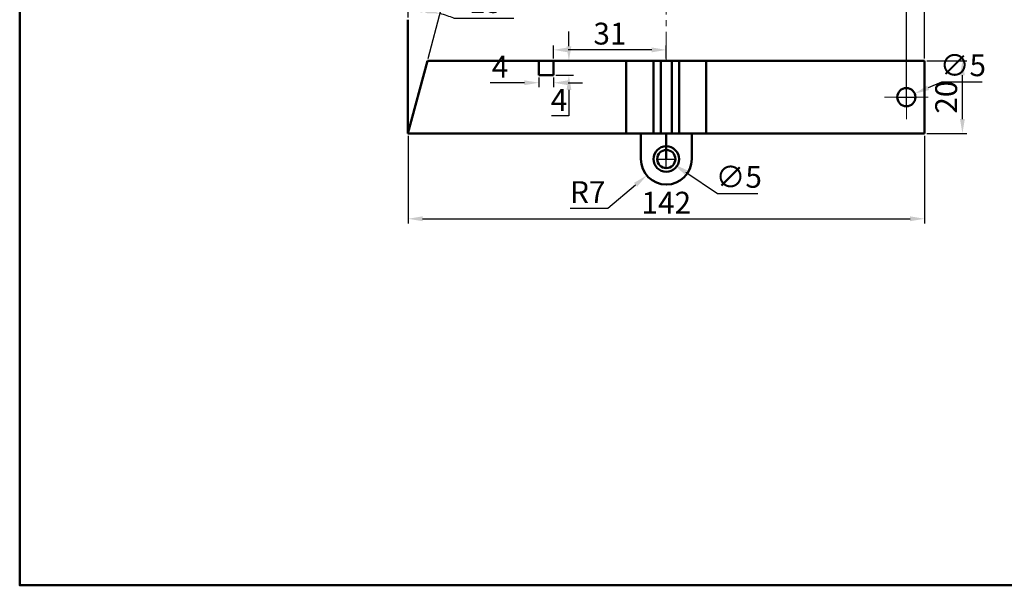
# Model space of a CAD drawing. Units: millimetres. Extents: x 1145 to 1687, y 12 to 400.
# Tile 1 of 6: x 1145 to 1416, y 12 to 168. Entities that reach past the tile are written whole.
import ezdxf

# ---------------------------------------------------------------- set-up
doc = ezdxf.new("R2010")
doc.units = ezdxf.units.MM
doc.header["$LTSCALE"] = 0.5
doc.linetypes.add('CENTER', pattern=[50.8, 31.75, -6.35, 6.35, -6.35])
for name, color, linetype, lineweight in [('M-CNTR', 1, 'CENTER', 18), ('M-DIMS', 2, 'Continuous', 25), ('M-OUTL', 7, 'Continuous', 50)]:
    doc.layers.add(name, color=color, linetype=linetype, lineweight=lineweight)
doc.styles.get("Standard").update_dxf_attribs({"font": 'arial.ttf'})
doc.dimstyles.new('ISO-25', dxfattribs={"dimtxt": 6, "dimasz": 4, "dimexe": 1.25, "dimexo": 0.625, "dimtad": 1, "dimtoh": 1, "dimdec": 0, "dimtxsty": 'Standard', "dimcen": 2.5, "dimadec": 0, "dimazin": 0, "dimtfac": 1, "dimtdec": 0, "dimtofl": 0, "dimtmove": 0, "dimatfit": 3, "dimfxl": 1, "dimarcsym": 0})

# ---------------------------------------------------------------- blocks, each defined once
blk = doc.blocks.new('*U65')
at = {"layer": 'M-CNTR', "color": 0, "transparency": 16777216}
for p, q in [((0, 0.5), (0, 6)), ((-6, 0), (-0.5, 0)), ((0.5, 0), (6, 0)), ((0, -6), (0, -0.5))]:
    blk.add_line(p, q, dxfattribs=at)
at = {"layer": 'M-CNTR', "color": 0, "linetype": 'Continuous', "transparency": 16777216}
for p, q in [((-0.25, 0), (0.25, 0)), ((0, -0.25), (0, 0.25))]:
    blk.add_line(p, q, dxfattribs=at)
blk = doc.blocks.new('*D69')
at = {"layer": 'Defpoints', "color": 0, "ltscale": 0.5, "transparency": 16777216}
for p in [(1321, 130.71), (1325.14, 127.91)]:
    blk.add_point(p, dxfattribs=at)
at = {"layer": 'M-DIMS', "color": 0, "lineweight": -2, "ltscale": 0.5, "transparency": 16777216}
for p, q in [((1323.07, 126.81), (1323.07, 131.81)), ((1320.57, 129.31), (1325.57, 129.31)), ((1337.11, 119.79), (1328.45, 125.66)), ((1348.24, 119.79), (1337.11, 119.79))]:
    blk.add_line(p, q, dxfattribs=at)
at = {"layer": 'M-DIMS', "color": 0, "ltscale": 0.5, "transparency": 16777216}
blk.add_solid([(1328.82, 126.22), (1328.07, 125.11), (1325.14, 127.91)], dxfattribs=at)
at = {"layer": 'M-DIMS', "color": 0, "ltscale": 0.5, "transparency": 16777216, "insert": (1342.99, 123.65), "char_height": 6, "attachment_point": 5}
blk.add_mtext('∅5', dxfattribs=at)
blk = doc.blocks.new('*D70')
at = {"layer": 'Defpoints', "color": 0, "ltscale": 0.5, "transparency": 16777216}
for p in [(1323.07, 129.31), (1317.7, 124.82)]:
    blk.add_point(p, dxfattribs=at)
at = {"layer": 'M-DIMS', "color": 0, "lineweight": -2, "ltscale": 0.5, "transparency": 16777216}
for p, q in [((1323.07, 126.81), (1323.07, 131.81)), ((1320.57, 129.31), (1325.57, 129.31)), ((1306.96, 115.84), (1314.63, 122.25)), ((1296.66, 115.84), (1306.96, 115.84))]:
    blk.add_line(p, q, dxfattribs=at)
at = {"layer": 'M-DIMS', "color": 0, "ltscale": 0.5, "transparency": 16777216}
blk.add_solid([(1314.2, 122.77), (1315.05, 121.74), (1317.7, 124.82)], dxfattribs=at)
at = {"layer": 'M-DIMS', "color": 0, "ltscale": 0.5, "transparency": 16777216, "insert": (1301.49, 119.46), "char_height": 6, "attachment_point": 5}
blk.add_mtext('R7', dxfattribs=at)
blk = doc.blocks.new('*D73')
at = {"layer": 'Defpoints', "color": 0, "ltscale": 0.5, "transparency": 16777216}
for p in [(1255.04, 170.27), (1252.07, 167.52), (1257.42, 156.31), (1252.07, 136.31), (1252.07, 136.31)]:
    blk.add_point(p, dxfattribs=at)
at = {"layer": 'M-DIMS', "color": 0, "lineweight": -2, "ltscale": 0.5, "transparency": 16777216}
for p, q in [((1252.07, 168.14), (1252.07, 171.65)), ((1257.59, 156.91), (1261.21, 170.44)), ((1264.68, 167.98), (1281.14, 167.98))]:
    blk.add_line(p, q, dxfattribs=at)
for start, end in [(81.7274, 83.2726), (68.2726, 75)]:
    blk.add_arc((1252.07, 136.31), 34.09, start, end, dxfattribs=at)
at = {"layer": 'M-DIMS', "color": 0, "ltscale": 0.5, "transparency": 16777216}
for points in [[(1256.02, 169.5), (1256.1, 170.83), (1252.07, 170.4)], [(1257.1, 170.69), (1256.84, 169.39), (1260.89, 169.24)]]:
    blk.add_solid(points, dxfattribs=at)
at = {"layer": 'M-DIMS', "color": 0, "ltscale": 0.5, "transparency": 16777216, "insert": (1274.91, 171.66), "char_height": 6, "attachment_point": 5}
blk.add_mtext('15°', dxfattribs=at)
blk = doc.blocks.new('*D74')
at = {"layer": 'Defpoints', "color": 0, "ltscale": 0.5, "transparency": 16777216}
for p in [(1292.07, 159.29), (1292.07, 156.31), (1323.07, 156.31)]:
    blk.add_point(p, dxfattribs=at)
at = {"layer": 'M-DIMS', "color": 0, "lineweight": -2, "ltscale": 0.5, "transparency": 16777216}
for p, q in [((1292.07, 156.94), (1292.07, 160.54)), ((1323.07, 156.94), (1323.07, 160.54)), ((1319.07, 159.29), (1296.07, 159.29))]:
    blk.add_line(p, q, dxfattribs=at)
at = {"layer": 'M-DIMS', "color": 0, "ltscale": 0.5, "transparency": 16777216}
for points in [[(1296.07, 159.96), (1296.07, 158.62), (1292.07, 159.29)], [(1319.07, 159.96), (1319.07, 158.62), (1323.07, 159.29)]]:
    blk.add_solid(points, dxfattribs=at)
at = {"layer": 'M-DIMS', "color": 0, "ltscale": 0.5, "transparency": 16777216, "insert": (1307.57, 162.98), "char_height": 6, "attachment_point": 5}
blk.add_mtext('31', dxfattribs=at)
blk = doc.blocks.new('*D75')
at = {"layer": 'Defpoints', "color": 0, "ltscale": 0.5, "transparency": 16777216}
for p in [(1292.07, 156.31), (1292.07, 152.31), (1296.3, 152.31)]:
    blk.add_point(p, dxfattribs=at)
at = {"layer": 'M-DIMS', "color": 0, "lineweight": -2, "ltscale": 0.5, "transparency": 16777216}
for p, q in [((1296.3, 160.31), (1296.3, 164.31)), ((1292.69, 156.31), (1297.55, 156.31)), ((1292.69, 152.31), (1297.55, 152.31)), ((1296.3, 148.31), (1296.3, 141.14)), ((1296.3, 141.14), (1291.53, 141.14))]:
    blk.add_line(p, q, dxfattribs=at)
at = {"layer": 'M-DIMS', "color": 0, "ltscale": 0.5, "transparency": 16777216}
for points in [[(1295.64, 160.31), (1296.97, 160.31), (1296.3, 156.31)], [(1295.64, 148.31), (1296.97, 148.31), (1296.3, 152.31)]]:
    blk.add_solid(points, dxfattribs=at)
at = {"layer": 'M-DIMS', "color": 0, "ltscale": 0.5, "transparency": 16777216, "insert": (1293.6, 144.76), "char_height": 6, "attachment_point": 5}
blk.add_mtext('4', dxfattribs=at)
blk = doc.blocks.new('*D76')
at = {"layer": 'Defpoints', "color": 0, "ltscale": 0.5, "transparency": 16777216}
for p in [(1288.07, 152.31), (1292.07, 152.31), (1288.07, 150.27)]:
    blk.add_point(p, dxfattribs=at)
at = {"layer": 'M-DIMS', "color": 0, "lineweight": -2, "ltscale": 0.5, "transparency": 16777216}
for p, q in [((1288.07, 151.69), (1288.07, 149.02)), ((1292.07, 151.69), (1292.07, 149.02)), ((1284.07, 150.27), (1274.67, 150.27)), ((1296.07, 150.27), (1300.07, 150.27))]:
    blk.add_line(p, q, dxfattribs=at)
at = {"layer": 'M-DIMS', "color": 0, "ltscale": 0.5, "transparency": 16777216}
for points in [[(1284.07, 150.93), (1284.07, 149.6), (1288.07, 150.27)], [(1296.07, 150.93), (1296.07, 149.6), (1292.07, 150.27)]]:
    blk.add_solid(points, dxfattribs=at)
at = {"layer": 'M-DIMS', "color": 0, "ltscale": 0.5, "transparency": 16777216, "insert": (1277.37, 153.89), "char_height": 6, "attachment_point": 5}
blk.add_mtext('4', dxfattribs=at)
blk = doc.blocks.new('TERMINAL-LUG-END')
at = {"ltscale": 0.5}
for p, q in [((0, 7), (0, 14)), ((14, 7), (14, 14))]:
    blk.add_line(p, q, dxfattribs=at)
blk.add_arc((7, 7), 7, 180, 0, dxfattribs=at)
blk = doc.blocks.new('*D96')
at = {"layer": 'Defpoints', "color": 0, "ltscale": 0.5, "transparency": 16777216}
for p in [(1252.07, 136.31), (1394.07, 136.31), (1394.07, 112.91)]:
    blk.add_point(p, dxfattribs=at)
at = {"layer": 'M-DIMS', "color": 0, "lineweight": -2, "ltscale": 0.5, "transparency": 16777216}
for p, q in [((1252.07, 135.69), (1252.07, 111.66)), ((1394.07, 135.69), (1394.07, 111.66)), ((1256.07, 112.91), (1390.07, 112.91))]:
    blk.add_line(p, q, dxfattribs=at)
at = {"layer": 'M-DIMS', "color": 0, "ltscale": 0.5, "transparency": 16777216}
for points in [[(1256.07, 113.58), (1256.07, 112.24), (1252.07, 112.91)], [(1390.07, 113.58), (1390.07, 112.24), (1394.07, 112.91)]]:
    blk.add_solid(points, dxfattribs=at)
at = {"layer": 'M-DIMS', "color": 0, "ltscale": 0.5, "transparency": 16777216, "insert": (1323.07, 116.55), "char_height": 6, "attachment_point": 5}
blk.add_mtext('142', dxfattribs=at)
blk = doc.blocks.new('*D97')
at = {"layer": 'Defpoints', "color": 0, "ltscale": 0.5, "transparency": 16777216}
for p in [(1394.07, 156.31), (1404.47, 156.31), (1394.07, 136.31)]:
    blk.add_point(p, dxfattribs=at)
at = {"layer": 'M-DIMS', "color": 0, "lineweight": -2, "ltscale": 0.5, "transparency": 16777216}
for p, q in [((1394.69, 156.31), (1405.72, 156.31)), ((1404.47, 140.31), (1404.47, 152.31)), ((1394.69, 136.31), (1405.72, 136.31))]:
    blk.add_line(p, q, dxfattribs=at)
at = {"layer": 'M-DIMS', "color": 0, "ltscale": 0.5, "transparency": 16777216}
for points in [[(1403.8, 152.31), (1405.13, 152.31), (1404.47, 156.31)], [(1403.8, 140.31), (1405.13, 140.31), (1404.47, 136.31)]]:
    blk.add_solid(points, dxfattribs=at)
at = {"layer": 'M-DIMS', "color": 0, "ltscale": 0.5, "transparency": 16777216, "insert": (1400.78, 146.31), "char_height": 6, "attachment_point": 5, "rotation": 90}
blk.add_mtext('20', dxfattribs=at)
blk = doc.blocks.new('*D98')
at = {"layer": 'Defpoints', "color": 0, "ltscale": 0.5, "transparency": 16777216}
for p in [(1394.07, 231.87), (1394.07, 156.31), (1389.07, 146.81)]:
    blk.add_point(p, dxfattribs=at)
at = {"layer": 'M-DIMS', "color": 0, "lineweight": -2, "ltscale": 0.5, "transparency": 16777216}
for p, q in [((1389.07, 147.44), (1389.07, 233.12)), ((1394.07, 156.94), (1394.07, 233.12)), ((1385.07, 231.87), (1381.07, 231.87)), ((1398.07, 231.87), (1407.29, 231.87))]:
    blk.add_line(p, q, dxfattribs=at)
at = {"layer": 'M-DIMS', "color": 0, "ltscale": 0.5, "transparency": 16777216}
for points in [[(1385.07, 232.54), (1385.07, 231.2), (1389.07, 231.87)], [(1398.07, 232.54), (1398.07, 231.2), (1394.07, 231.87)]]:
    blk.add_solid(points, dxfattribs=at)
at = {"layer": 'M-DIMS', "color": 0, "ltscale": 0.5, "transparency": 16777216, "insert": (1404.68, 235.55), "char_height": 6, "attachment_point": 5}
blk.add_mtext('5', dxfattribs=at)
blk = doc.blocks.new('*D117')
at = {"layer": 'Defpoints', "color": 0, "ltscale": 0.5, "transparency": 16777216}
for p in [(1391.36, 147.29), (1386.77, 145.33)]:
    blk.add_point(p, dxfattribs=at)
at = {"layer": 'M-DIMS', "color": 0, "lineweight": -2, "ltscale": 0.5, "transparency": 16777216}
for p, q in [((1398.72, 150.43), (1395.04, 148.86)), ((1409.85, 150.43), (1398.72, 150.43)), ((1386.57, 146.31), (1391.57, 146.31)), ((1389.07, 143.81), (1389.07, 148.81))]:
    blk.add_line(p, q, dxfattribs=at)
at = {"layer": 'M-DIMS', "color": 0, "ltscale": 0.5, "transparency": 16777216}
blk.add_solid([(1394.78, 149.48), (1395.31, 148.25), (1391.36, 147.29)], dxfattribs=at)
at = {"layer": 'M-DIMS', "color": 0, "ltscale": 0.5, "transparency": 16777216, "insert": (1404.6, 154.29), "char_height": 6, "attachment_point": 5}
blk.add_mtext('∅5', dxfattribs=at)

msp = doc.modelspace()

# ---------------------------------------------------------------- linework, layer by layer
at = {"layer": 'M-CNTR', "ltscale": 0.5}
msp.add_line((1323.0658, 156.3102), (1323.0755, 214.3937), dxfattribs=at)
at = {"layer": 'M-OUTL', "ltscale": 0.5}
for p, q in [((1252.0658, 136.3102), (1252.0658, 167.5151)), ((1252.0658, 136.3102), (1257.4248, 156.3102)), ((1312.0658, 156.3102), (1257.4248, 156.3102)), ((1288.0658, 152.3102), (1288.0658, 156.3102)), ((1292.0658, 156.3102), (1292.0658, 152.3102)), ((1312.0658, 156.3102), (1312.0658, 136.3102)), ((1334.0658, 156.3102), (1312.0658, 156.3102)), ((1319.5658, 156.3102), (1319.5658, 136.3102)), ((1321.5658, 156.3102), (1321.5658, 136.3102)), ((1324.5658, 156.3102), (1324.5658, 136.3102)), ((1326.5658, 156.3102), (1326.5658, 136.3102)), ((1334.0658, 156.3102), (1334.0658, 136.3102)), ((1334.0658, 156.3102), (1394.0658, 156.3102)), ((1394.0658, 156.3102), (1394.0658, 136.3102)), ((1292.0658, 152.3102), (1288.0658, 152.3102)), ((1252.0658, 136.3102), (1312.0658, 136.3102)), ((1334.0658, 136.3102), (1312.0658, 136.3102)), ((1323.0658, 136.3102), (1323.0658, 129.3102)), ((1394.0658, 136.3102), (1334.0658, 136.3102))]:
    msp.add_line(p, q, dxfattribs=at)
msp.add_lwpolyline([(1145.3327, 400.1417), (1687.1285, 400.1417), (1687.1285, 12.2645), (1145.3327, 12.2645)], close=True, dxfattribs=at)
for centre, radius in [((1389.0658, 146.3102), 2.5), ((1323.0658, 129.3102), 3.5), ((1323.0658, 129.3102), 2.5)]:
    msp.add_circle(centre, radius, dxfattribs=at)

# ---------------------------------------------------------------- block references
at = {"layer": 'M-CNTR'}
msp.add_blockref('*U65', (1389.0658, 146.3102), dxfattribs=at)
at = {"layer": 'M-OUTL'}
msp.add_blockref('TERMINAL-LUG-END', (1316.0662, 122.3101), dxfattribs=at)

# ---------------------------------------------------------------- dimensions: what is measured, and where the dimension line sits
at = {"layer": 'M-DIMS', "ltscale": 0.5}
for base, p1, p2, override, picture, middle in [((1394.0658, 231.871), (1389.0658, 146.8102), (1394.0658, 156.3102), {"dimdec": 0, "dimlfac": 1, "dimrnd": 0, "dimzin": 0, "dimdsep": 46, "dimlunit": 2}, '*D98', (1404.6799, 235.5471)), ((1292.0658, 159.2885), (1323.0658, 156.3102), (1292.0658, 156.3102), {"dimclrd": 0, "dimclre": 0, "dimclrt": 0}, '*D74', (1307.5658, 162.979)), ((1288.0658, 150.2663), (1292.0658, 152.3102), (1288.0658, 152.3102), {"dimclrd": 0, "dimclre": 0, "dimclrt": 0}, '*D76', (1277.3658, 153.8913)), ((1394.0658, 112.9102), (1252.0658, 136.3102), (1394.0658, 136.3102), {"dimdec": 0, "dimlfac": 1, "dimrnd": 0, "dimzin": 0, "dimdsep": 46, "dimlunit": 2}, '*D96', (1323.0658, 116.5475))]:
    dim = msp.add_linear_dim(base=base, p1=p1, p2=p2, dimstyle='ISO-25', override=override, dxfattribs=at)
    dim.commit()
    dim.dimension.update_dxf_attribs({"geometry": picture, "text_midpoint": middle})
dim = msp.add_angular_dim_2l(base=(1255.0366, 170.267), line1=((1252.0658, 136.3102), (1257.4248, 156.3102)), line2=((1252.0658, 136.3102), (1252.0658, 167.5151)), dimstyle='ISO-25', override={"dimclrd": 0, "dimclre": 0, "dimclrt": 0}, dxfattribs=at)
dim.commit()
dim.dimension.update_dxf_attribs({"geometry": '*D73', "text_midpoint": (1274.9123, 171.6634)})
dim = msp.add_linear_dim(base=(1296.3041, 152.3102), p1=(1292.0658, 156.3102), p2=(1292.0658, 152.3102), angle=90, dimstyle='ISO-25', override={"dimclrd": 0, "dimclre": 0, "dimclrt": 0}, dxfattribs=at)
dim.commit()
dim.dimension.update_dxf_attribs({"geometry": '*D75', "text_midpoint": (1293.604, 141.135), "dimtype": 160})
dim = msp.add_diameter_dim_2p(p1=(1386.7668, 145.3281), p2=(1391.3648, 147.2923), dimstyle='ISO-25', override={"dimdec": 0, "dimlfac": 1, "dimrnd": 0, "dimzin": 0, "dimdsep": 46, "dimlunit": 2}, dxfattribs=at)
dim.commit()
dim.dimension.update_dxf_attribs({"geometry": '*D117', "text_midpoint": (1404.5998, 150.4349), "dimtype": 163})
dim = msp.add_linear_dim(base=(1404.4658, 156.3102), p1=(1394.0658, 136.3102), p2=(1394.0658, 156.3102), angle=90, dimstyle='ISO-25', override={"dimdec": 0, "dimlfac": 1, "dimrnd": 0, "dimzin": 0, "dimdsep": 46, "dimlunit": 2}, dxfattribs=at)
dim.commit()
dim.dimension.update_dxf_attribs({"geometry": '*D97', "text_midpoint": (1400.7773, 146.3102)})
dim = msp.add_radius_dim(center=(1323.0658, 129.3102), mpoint=(1317.6958, 124.8198), dimstyle='ISO-25', override={"dimclrd": 0, "dimclre": 0, "dimclrt": 0}, dxfattribs=at)
dim.commit()
dim.dimension.update_dxf_attribs({"geometry": '*D70', "text_midpoint": (1301.4932, 119.464)})
dim = msp.add_diameter_dim_2p(p1=(1320.9963, 130.7127), p2=(1325.1353, 127.9076), dimstyle='ISO-25', override={"dimclrd": 0, "dimclre": 0, "dimclrt": 0}, dxfattribs=at)
dim.commit()
dim.dimension.update_dxf_attribs({"geometry": '*D69', "text_midpoint": (1342.9854, 123.6501)})

doc.saveas('drawing.dxf')
